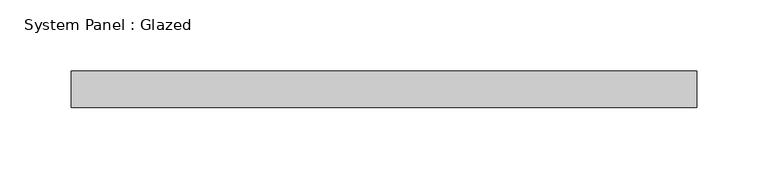
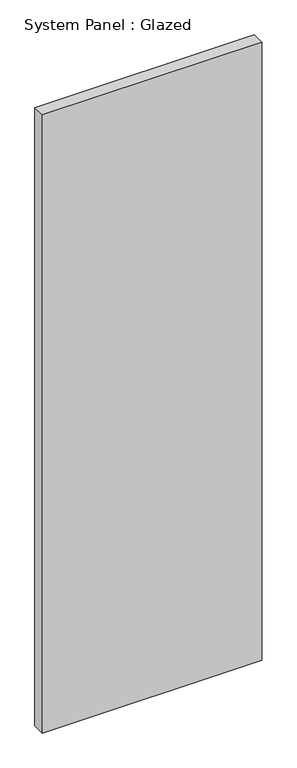
"""IFC4 building model written with IfcOpenShell, lengths in millimetres: plate geometry, System Panel : Glazed."""

from ifc_helpers import new_model, si_unit, origin, origin_with_axes, place, context, project, spatial, polyline, outline, extrude, source, transform, mapped, element, save


def system_panel_glazed_197f3525(model_context):
    return source(origin(), model_context, "Body", "SweptSolid", [
        extrude(outline(polyline([(219.075, 19.05), (-219.075, 19.05), (-219.075, 44.45), (219.075, 44.45), (219.075, 19.05)])), origin_with_axes(), (0.0, 0.0, 1.0), 1305.2179754),
    ])


if __name__ == "__main__":
    model = new_model("IFC4")
    model_context = context("Model", 3, world=origin())
    ifc_project = project(units=[si_unit("LENGTHUNIT", "METRE", prefix="MILLI")], contexts=[model_context])
    site = spatial("IfcSite", under=ifc_project)
    building = spatial("IfcBuilding", under=site)
    placement = place(None, origin())
    system_panel_glazed_shape = system_panel_glazed_197f3525(model_context)
    element("IfcPlate", 1, ObjectType="System Panel : Glazed", at=placement, inside=building, context=model_context, shape_type="MappedRepresentation", body=[
        mapped(system_panel_glazed_shape, transform((0.0, 0.0, 0.0), x_axis=(1.0, 0.0, 0.0), y_axis=(0.0, 1.0, 0.0), z_axis=(0.0, 0.0, 1.0))),
    ])
    save(model, "model.ifc")

# Revit data of these elements
# Type "System Panel : Glazed"
#   Construction Type Id = "GSP4R"
#   Analytic Construction = "1/8 in Pilkington single glazing"
#   Visual Light Transmittance = 0.9
#   Solar Heat Gain Coefficient = 0.86
#   Heat Transfer Coefficient (U) = 1.18115 BTU/(h·ft²·°F)
#   Define Thermal Properties by = 1
# Element 1 (IfcPlate, "System Panel : Glazed")
#   Materials on its faces: "Glass"
# Materials
#   "Glass": class "Glass", colour RGB 0 128 192, transparency 0.75, Description = "Soda Lime Glass", Cost = 0
